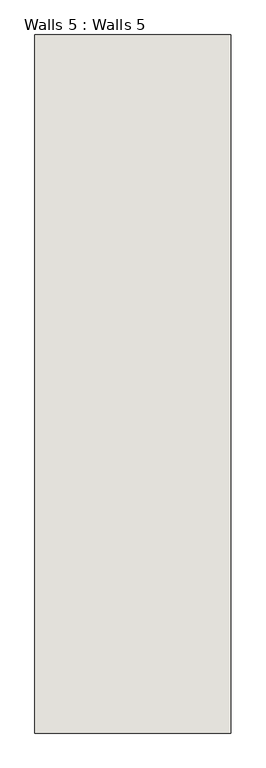
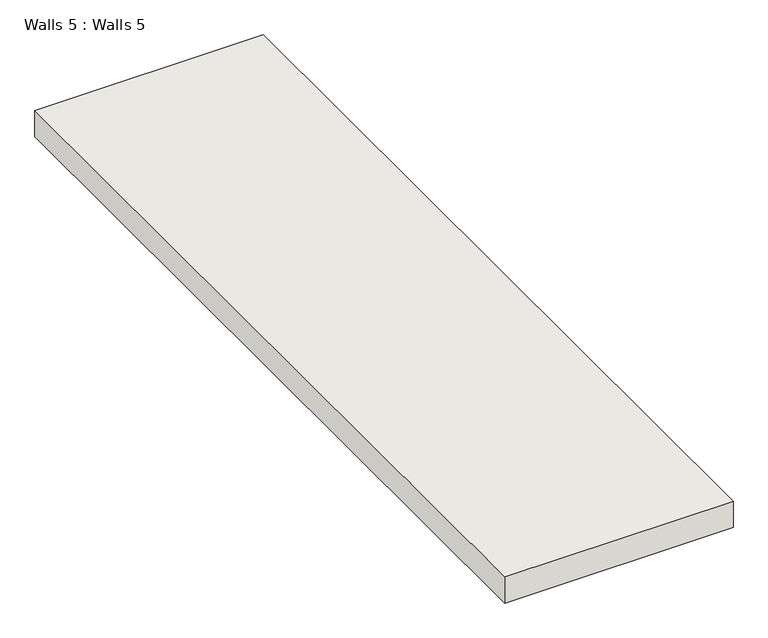
"""IFC4 building model written with IfcOpenShell, lengths in millimetres: wall geometry, Walls 5 : Walls 5."""

from ifc_helpers import new_model, si_unit, frame, origin, place, context, project, spatial, polyline, outline, extrude, source, transform, mapped, element, save


def walls_5_walls_5_8fe41d8f(model_context):
    return source(origin(), model_context, "Body", "SweptSolid", [
        extrude(outline(polyline([(-15693.0519043, -1845.8046854), (-15693.0519043, -3390.9180898), (-16126.4519043, -3390.9180898), (-16126.4519043, -1845.8046854), (-15693.0519043, -1845.8046854)])), frame((0.0, 0.0, 2762.6009455), z_axis=(0.0, 0.0, 1.0), x_axis=(1.0, 0.0, 0.0)), (0.0, 0.0, 1.0), 52.693252),
    ])


if __name__ == "__main__":
    model = new_model("IFC4")
    model_context = context("Model", 3, world=origin())
    ifc_project = project(units=[si_unit("LENGTHUNIT", "METRE", prefix="MILLI")], contexts=[model_context])
    site = spatial("IfcSite", under=ifc_project)
    building = spatial("IfcBuilding", under=site)
    placement = place(None, origin())
    walls_5_walls_5_shape = walls_5_walls_5_8fe41d8f(model_context)
    element("IfcWall", 1, ObjectType="Walls 5 : Walls 5", at=placement, inside=building, context=model_context, shape_type="MappedRepresentation", body=[
        mapped(walls_5_walls_5_shape, transform((0.0, 0.0, 0.0), x_axis=(1.0, 0.0, 0.0), y_axis=(0.0, 1.0, 0.0), z_axis=(0.0, 0.0, 1.0))),
    ])
    save(model, "model.ifc")

# Revit data of these elements
# Element 1 (IfcWall, "Walls 5 : Walls 5")
#   Materials on its faces: "Default Wall"
# Materials
#   "Default Wall": colour RGB 80 80 80, transparency 0
